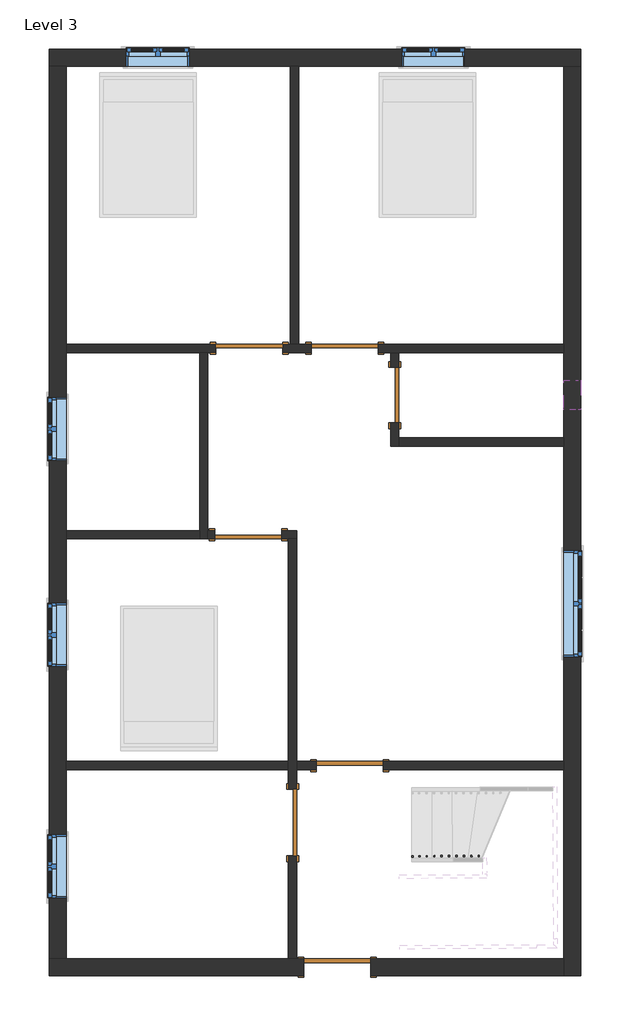
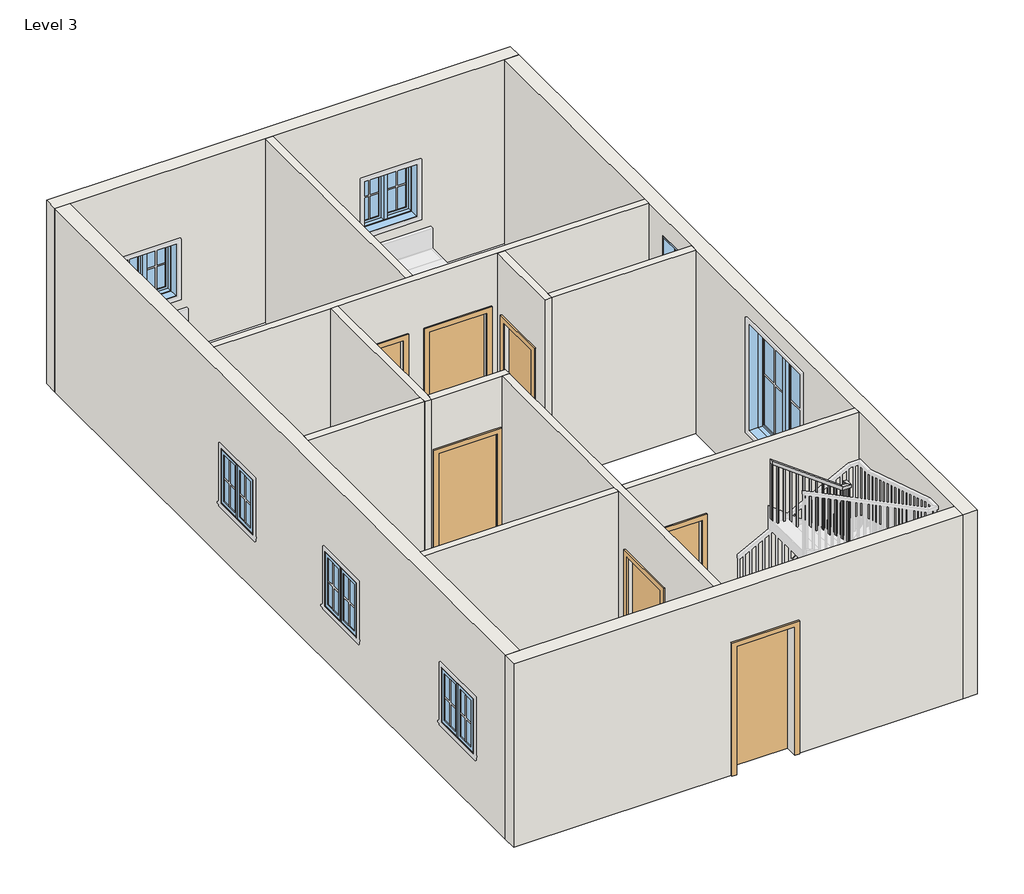
# One storey, part 1 of 2: 13 walls, 7 doors, 7 windows, 1 railing.
"""IFC4 building model written with IfcOpenShell, lengths in millimetres."""

from ifc_helpers import new_model, si_unit, frame, origin, place, context, project, spatial, polyline, outline, extrude, faceted_brep, transform, mapped, element, save
from components import door_f2b275c1, door_e5f9f3c4, door_305aa2a5, door_a90ba1ad, window_aa618e30, window_339605e1, window_9ac97e1a

model = new_model("IFC4")

# Units and contexts
model_context = context("Model", 3, world=origin())
ifc_project = project(units=[si_unit("LENGTHUNIT", "METRE", prefix="MILLI")], contexts=[model_context])

# Site, building, storey
site = spatial("IfcSite", under=ifc_project)
building = spatial("IfcBuilding", under=site)
storey = spatial("IfcBuildingStorey", under=building, Name="Level 3", Elevation=3200.4)

# Doors
placement = place(None, origin())
door_shape = door_f2b275c1(model_context)
element("IfcDoor", 1, ObjectType="Single-Flush : 30\" x 80\"", at=placement, inside=storey, context=model_context, shape_type="MappedRepresentation", body=[
    mapped(door_shape, transform((-163.0415084, 2144.7435985, 3200.4), x_axis=(0.0, 1.0, 0.0), y_axis=(-1.0, 0.0, 0.0), z_axis=(0.0, 0.0, 1.0))),
])
door_2_shape = door_e5f9f3c4(model_context)
element("IfcDoor", 2, ObjectType="Single-Flush : 36\" x 84\"", at=placement, inside=storey, context=model_context, shape_type="MappedRepresentation", body=[
    mapped(door_2_shape, transform((-2156.9415084, 2786.0935985, 3200.4), x_axis=(1.0, 0.0, 0.0), y_axis=(0.0, 1.0, 0.0), z_axis=(0.0, 0.0, 1.0))),
])
door_3_shape = door_305aa2a5(model_context)
element("IfcDoor", 3, ObjectType="Single-Flush : 36\" x 84\"", at=placement, inside=storey, context=model_context, shape_type="MappedRepresentation", body=[
    mapped(door_3_shape, transform((-848.8415084, 2786.0935985, 3200.4), x_axis=(-1.0, 0.0, 0.0), y_axis=(0.0, -1.0, 0.0), z_axis=(0.0, 0.0, 1.0))),
])
element("IfcDoor", 4, ObjectType="Single-Flush : 36\" x 84\"", at=placement, inside=storey, context=model_context, shape_type="MappedRepresentation", body=[
    mapped(door_3_shape, transform((-2170.1582019, 233.3935985, 3200.4), x_axis=(1.0, 0.0, 0.0), y_axis=(0.0, 1.0, 0.0), z_axis=(0.0, 0.0, 1.0))),
])
element("IfcDoor", 5, ObjectType="Single-Flush : 36\" x 84\"", at=placement, inside=storey, context=model_context, shape_type="MappedRepresentation", body=[
    mapped(door_3_shape, transform((-778.9915084, -2928.9064015, 3200.4), x_axis=(-1.0, 0.0, 0.0), y_axis=(0.0, -1.0, 0.0), z_axis=(0.0, 0.0, 1.0))),
])
element("IfcDoor", 6, ObjectType="Single-Flush : 36\" x 84\"", at=placement, inside=storey, context=model_context, shape_type="MappedRepresentation", body=[
    mapped(door_3_shape, transform((-1561.0748955, -3709.9564015, 3200.4), x_axis=(0.0, 1.0, 0.0), y_axis=(-1.0, 0.0, 0.0), z_axis=(0.0, 0.0, 1.0))),
])
door_4_shape = door_a90ba1ad(model_context)
element("IfcDoor", 7, ObjectType="Single-Flush : 36\" x 84\"", at=placement, inside=storey, context=model_context, shape_type="MappedRepresentation", body=[
    mapped(door_4_shape, transform((-951.4748955, -5691.1564015, 3200.4), x_axis=(-1.0, 0.0, 0.0), y_axis=(0.0, -1.0, 0.0), z_axis=(0.0, 0.0, 1.0))),
])

# Railing
element("IfcRailing", 8, ObjectType="Handrail - Rectangular", at=placement, inside=storey, context=model_context, shape_type="SolidModel", body=[
    faceted_brep([(73.2591805, -4146.3303197, 4792.1333333), (73.2591805, -4146.3303197, 4725.5495342), (73.5214139, -4197.1296428, 4725.5495342), (73.5214139, -4197.1296428, 4792.1333333), (1064.2769136, -4141.2145447, 5631.8511215), (1082.90463, -4141.1183857, 5581.0511215), (1083.1668634, -4191.9177089, 5581.0511215), (1064.5391469, -4192.0138678, 5631.8511215), (1144.655904, -4140.7996168, 5631.8511215), (1144.9181373, -4191.59894, 5631.8511215), (1144.9181373, -4191.59894, 5581.0511215), (1144.655904, -4140.7996168, 5581.0511215)], [[[0, 1, 2, 3]], [[1, 0, 4, 5]], [[2, 1, 5, 6]], [[3, 2, 6, 7]], [[0, 3, 7, 4]], [[8, 9, 10, 11]], [[5, 4, 8, 11]], [[6, 5, 11, 10]], [[7, 6, 10, 9]], [[4, 7, 9, 8]]]),
    faceted_brep([(1144.9181373, -4191.59894, 5640.3305642), (1144.9181373, -4191.59894, 5519.048826), (1094.1188142, -4191.8611734, 5519.048826), (1094.1188142, -4191.8611734, 5640.3305642), (1145.9670708, -4394.7962326, 6080.8506209), (1146.2293041, -4445.5955558, 6069.6988968), (1095.429981, -4445.8577892, 6069.6988968), (1095.1677476, -4395.058466, 6080.8506209), (1145.9670708, -4394.7962326, 6331.4424257), (1146.2293041, -4445.5955558, 6280.6424257), (1095.429981, -4445.8577892, 6280.6424257), (1095.1677476, -4395.058466, 6331.4424257), (1146.6226542, -4521.7945406, 6331.4424257), (1146.6226542, -4521.7945406, 6280.6424257), (1095.5610976, -4471.2574507, 6280.6424257), (1095.5610976, -4471.2574507, 6331.4424257), (1019.6243463, -4522.4501239, 6331.4424257), (1002.8333893, -4522.5368013, 6280.6424257), (1002.5711559, -4471.7374781, 6280.6424257), (1019.3621129, -4471.6508008, 6331.4424257), (-100.5579777, -4528.232665, 7162.8), (-100.8202111, -4477.4333418, 7162.8), (-100.8202111, -4477.4333418, 7099.5383775), (-100.5579777, -4528.232665, 7099.5383775)], [[[0, 1, 2, 3]], [[1, 0, 4, 5]], [[2, 1, 5, 6]], [[3, 2, 6, 7]], [[0, 3, 7, 4]], [[5, 4, 8, 9]], [[6, 5, 9, 10]], [[7, 6, 10, 11]], [[4, 7, 11, 8]], [[9, 8, 12, 13]], [[10, 9, 13, 14]], [[11, 10, 14, 15]], [[8, 11, 15, 12]], [[13, 12, 16, 17]], [[14, 13, 17, 18]], [[15, 14, 18, 19]], [[12, 15, 19, 16]], [[20, 21, 22, 23]], [[17, 16, 20, 23]], [[18, 17, 23, 22]], [[19, 18, 22, 21]], [[16, 19, 21, 20]]]),
    extrude(outline(polyline([(235.6690058, -19.05), (221.5309941, 0.0), (1247.144155, 0.0), (1247.144155, -19.05), (235.6690058, -19.05)])), frame((-107.5675843, -4512.3936381, 7326.2108217), z_axis=(-0.005162073969672187, 0.9999866764074069, 0.0), x_axis=(0.0, 0.0, -1.0)), (0.0, 0.0, 1.0), 19.05),
    extrude(outline(polyline([(235.6690059, -19.05), (221.5309942, 0.0), (1171.7414261, 0.0), (1171.7414261, -19.05), (235.6690059, -19.05)])), frame((-5.968938, -4511.8691714, 7250.8080928), z_axis=(-0.005162073969672187, 0.9999866764074069, 0.0), x_axis=(0.0, 0.0, -1.0)), (0.0, 0.0, 1.0), 19.05),
    extrude(outline(polyline([(235.6690058, -19.05), (221.5309941, 0.0), (1096.3386971, 0.0), (1096.3386971, -19.05), (235.6690058, -19.05)])), frame((95.6297083, -4511.3447046, 7175.4053638), z_axis=(-0.005162073969672187, 0.9999866764074069, 0.0), x_axis=(0.0, 0.0, -1.0)), (0.0, 0.0, 1.0), 19.05),
    extrude(outline(polyline([(235.6690059, -19.0499999), (221.5309942, 0.0), (1190.2693016, 0.0), (1190.2693016, -19.0499999), (235.6690059, -19.0499999)])), frame((197.2283547, -4510.8202379, 7100.0026349), z_axis=(-0.005162073969672187, 0.9999866764074069, 0.0), x_axis=(0.0, 0.0, -1.0)), (0.0, 0.0, 1.0), 19.05),
    extrude(outline(polyline([(235.6690058, -19.05), (221.5309942, 0.0), (1114.8665726, 0.0), (1114.8665726, -19.05), (235.6690058, -19.05)])), frame((298.827001, -4510.2957712, 7024.5999059), z_axis=(-0.005162073969672187, 0.9999866764074069, 0.0), x_axis=(0.0, 0.0, -1.0)), (0.0, 0.0, 1.0), 19.05),
    extrude(outline(polyline([(235.6690058, -19.05), (221.5309941, 0.0), (1039.4638436, 0.0), (1039.4638436, -19.05), (235.6690058, -19.05)])), frame((400.4256473, -4509.7713045, 6949.1971769), z_axis=(-0.005162073969672187, 0.9999866764074069, 0.0), x_axis=(0.0, 0.0, -1.0)), (0.0, 0.0, 1.0), 19.05),
    extrude(outline(polyline([(235.6690058, -19.05), (221.5309942, 0.0), (1133.394448, 0.0), (1133.394448, -19.05), (235.6690058, -19.05)])), frame((502.0242936, -4509.2468378, 6873.794448), z_axis=(-0.005162073969672187, 0.9999866764074069, 0.0), x_axis=(0.0, 0.0, -1.0)), (0.0, 0.0, 1.0), 19.05),
    extrude(outline(polyline([(235.6690058, -19.05), (221.5309941, 0.0), (1057.991719, 0.0), (1057.991719, -19.05), (235.6690058, -19.05)])), frame((603.6229399, -4508.7223711, 6798.391719), z_axis=(-0.005162073969672187, 0.9999866764074069, 0.0), x_axis=(0.0, 0.0, -1.0)), (0.0, 0.0, 1.0), 19.05),
    extrude(outline(polyline([(235.6690059, -19.05), (221.5309942, 0.0), (1151.9223234, 0.0), (1151.9223234, -19.05), (235.6690059, -19.05)])), frame((705.2215863, -4508.1979044, 6722.9889901), z_axis=(-0.005162073969672187, 0.9999866764074069, 0.0), x_axis=(0.0, 0.0, -1.0)), (0.0, 0.0, 1.0), 19.05),
    extrude(outline(polyline([(235.6690058, -19.05), (221.5309941, 0.0), (1076.5195944, 0.0), (1076.5195944, -19.05), (235.6690058, -19.05)])), frame((806.8202326, -4507.6734376, 6647.5862611), z_axis=(-0.005162073969672187, 0.9999866764074069, 0.0), x_axis=(0.0, 0.0, -1.0)), (0.0, 0.0, 1.0), 19.05),
    extrude(outline(polyline([(235.6690059, -19.05), (221.5309942, 0.0), (1170.4501989, 0.0), (1170.4501989, -19.05), (235.6690059, -19.05)])), frame((908.4188789, -4507.1489709, 6572.1835322), z_axis=(-0.005162073969672187, 0.9999866764074069, 0.0), x_axis=(0.0, 0.0, -1.0)), (0.0, 0.0, 1.0), 19.05),
    extrude(outline(polyline([(235.6690058, -19.05), (221.5309942, 0.0), (1095.0474699, 0.0), (1095.0474699, -19.05), (235.6690058, -19.05)])), frame((1010.0175252, -4506.6245042, 6496.7808032), z_axis=(-0.005162073969672187, 0.9999866764074069, 0.0), x_axis=(0.0, 0.0, -1.0)), (0.0, 0.0, 1.0), 19.05),
    extrude(outline(polyline([(1111.3867174, -4461.6506297), (1130.4364636, -4461.5522922), (1130.5348011, -4480.6020384), (1111.4850549, -4480.7003759), (1111.3867174, -4461.6506297)])), frame((0.0, 0.0, 5232.4), z_axis=(0.0, 0.0, 1.0), x_axis=(1.0, 0.0, 0.0)), (0.0, 0.0, 1.0), 1048.2424257),
    extrude(outline(polyline([(207.9506224, -19.05), (249.2493777, 0.0), (1070.0372089, 0.0), (1070.0372089, -19.05), (207.9506224, -19.05)])), frame((1110.8622507, -4360.0519834, 6133.1038756), z_axis=(0.9999866764074068, 0.005162073969671281, 0.0), x_axis=(0.0, 0.0, -1.0)), (0.0, 0.0, 1.0), 19.05),
    extrude(outline(polyline([(207.9506224, -19.05), (249.2493777, 0.0), (1019.110514, 0.0), (1019.110514, -19.05), (207.9506224, -19.05)])), frame((1110.3377839, -4258.4533371, 5912.8438473), z_axis=(0.9999866764074068, 0.005162073969671281, 0.0), x_axis=(0.0, 0.0, -1.0)), (0.0, 0.0, 1.0), 19.05),
    extrude(outline(polyline([(1079.9010561, -4176.0593559), (1079.8027186, -4157.0096098), (1098.8524648, -4156.9112722), (1098.9508023, -4175.9610184), (1079.9010561, -4176.0593559)])), frame((0.0, 0.0, 4555.0666667), z_axis=(0.0, 0.0, 1.0), x_axis=(1.0, 0.0, 0.0)), (0.0, 0.0, 1.0), 1025.9844548),
    extrude(outline(polyline([(220.5293015, -19.05), (236.6706986, 0.0), (1343.2032603, 0.0), (1343.2032603, -19.05), (220.5293015, -19.05)])), frame((978.3024098, -4176.5838227, 5728.9365936), z_axis=(-0.005162073969671482, 0.9999866764074068, 0.0), x_axis=(0.0, 0.0, -1.0)), (0.0, 0.0, 1.0), 19.05),
    extrude(outline(polyline([(220.5293015, -19.05), (236.6706985, 0.0), (1257.1158092, 0.0), (1257.1158092, -19.05), (220.5293015, -19.05)])), frame((876.7037635, -4177.1082894, 5642.8491425), z_axis=(-0.005162073969671482, 0.9999866764074068, 0.0), x_axis=(0.0, 0.0, -1.0)), (0.0, 0.0, 1.0), 19.05),
    extrude(outline(polyline([(220.5293015, -19.05), (236.6706986, 0.0), (1340.3616915, 0.0), (1340.3616915, -19.05), (220.5293015, -19.05)])), frame((775.1051171, -4177.6327561, 5556.7616915), z_axis=(-0.005162073969671482, 0.9999866764074068, 0.0), x_axis=(0.0, 0.0, -1.0)), (0.0, 0.0, 1.0), 19.05),
    extrude(outline(polyline([(220.5293014, -19.05), (236.6706985, 0.0), (1254.2742404, 0.0), (1254.2742404, -19.05), (220.5293014, -19.05)])), frame((673.5064708, -4178.1572228, 5470.6742404), z_axis=(-0.005162073969671482, 0.9999866764074068, 0.0), x_axis=(0.0, 0.0, -1.0)), (0.0, 0.0, 1.0), 19.05),
    extrude(outline(polyline([(220.5293015, -19.05), (236.6706985, 0.0), (1337.5201227, 0.0), (1337.5201227, -19.05), (220.5293015, -19.05)])), frame((571.9078245, -4178.6816895, 5384.5867894), z_axis=(-0.005162073969671482, 0.9999866764074068, 0.0), x_axis=(0.0, 0.0, -1.0)), (0.0, 0.0, 1.0), 19.05),
    extrude(outline(polyline([(220.5293015, -19.05), (236.6706986, 0.0), (1251.4326717, 0.0), (1251.4326717, -19.05), (220.5293015, -19.05)])), frame((470.3091782, -4179.2061562, 5298.4993384), z_axis=(-0.005162073969671482, 0.9999866764074068, 0.0), x_axis=(0.0, 0.0, -1.0)), (0.0, 0.0, 1.0), 19.05),
    extrude(outline(polyline([(220.5293014, -19.0499999), (236.6706985, 0.0), (1165.3452206, 0.0), (1165.3452206, -19.0499999), (220.5293014, -19.0499999)])), frame((368.7105319, -4179.7306229, 5212.4118873), z_axis=(-0.005162073969671482, 0.9999866764074068, 0.0), x_axis=(0.0, 0.0, -1.0)), (0.0, 0.0, 1.0), 19.05),
    extrude(outline(polyline([(220.5293015, -19.05), (236.6706986, 0.0), (1248.591103, 0.0), (1248.591103, -19.05), (220.5293015, -19.05)])), frame((267.1118855, -4180.2550897, 5126.3244363), z_axis=(-0.005162073969671482, 0.9999866764074068, 0.0), x_axis=(0.0, 0.0, -1.0)), (0.0, 0.0, 1.0), 19.05),
    extrude(outline(polyline([(220.5293014, -19.05), (236.6706985, 0.0), (1162.5036519, 0.0), (1162.5036519, -19.05), (220.5293014, -19.05)])), frame((165.5132392, -4180.7795564, 5040.2369852), z_axis=(-0.005162073969671482, 0.9999866764074068, 0.0), x_axis=(0.0, 0.0, -1.0)), (0.0, 0.0, 1.0), 19.05),
    extrude(outline(polyline([(1111.5178341, -4487.0502913), (1130.5675802, -4486.9519538), (1130.6659177, -4506.0017), (1111.6161716, -4506.1000375), (1111.5178341, -4487.0502913)])), frame((0.0, 0.0, 5232.4), z_axis=(0.0, 0.0, 1.0), x_axis=(1.0, 0.0, 0.0)), (0.0, 0.0, 1.0), 1048.2424257),
    extrude(outline(polyline([(1109.9116547, -4175.9044369), (1109.8133172, -4156.8546908), (1128.8630634, -4156.7563533), (1128.9614009, -4175.8060994), (1109.9116547, -4175.9044369)])), frame((0.0, 0.0, 4724.4), z_axis=(0.0, 0.0, 1.0), x_axis=(1.0, 0.0, 0.0)), (0.0, 0.0, 1.0), 856.6511215),
    extrude(outline(polyline([(235.6690058, -19.05), (221.5309941, 0.0), (1242.0027049, 0.0), (1242.0027049, -19.05), (235.6690058, -19.05)])), frame((-100.6399256, -4512.3578765, 7321.0693716), z_axis=(-0.005162073969672187, 0.9999866764074069, 0.0), x_axis=(0.0, 0.0, -1.0)), (0.0, 0.0, 1.0), 19.05),
    extrude(outline(polyline([(220.5293014, -19.05), (236.6706985, 0.0), (1084.4868994, 0.0), (1084.4868994, -19.05), (220.5293014, -19.05)])), frame((73.439466, -4181.2548543, 4962.2202327), z_axis=(-0.005162073969671482, 0.9999866764074068, 0.0), x_axis=(0.0, 0.0, -1.0)), (0.0, 0.0, 1.0), 19.05),
])

# Walls
element("IfcWall", 9, ObjectType="WALL4.5\"", at=placement, inside=storey, context=model_context, shape_type="Brep", body=[
    faceted_brep([(-1699.7415084, 2728.9435985, 3200.4), (-1306.0415084, 2728.9435985, 3200.4), (-1306.0415084, 2728.9435985, 5334.0), (-391.6415084, 2728.9435985, 5334.0), (-391.6415084, 2728.9435985, 3200.4), (-220.1915084, 2728.9435985, 3200.4), (-105.8915084, 2728.9435985, 3200.4), (2154.7084916, 2728.9435985, 3200.4), (2154.7084916, 2728.9435985, 6248.4), (-105.8915084, 2728.9435985, 6248.4), (-220.1915084, 2728.9435985, 6248.4), (-2722.0915084, 2728.9435985, 6248.4), (-2836.3915084, 2728.9435985, 6248.4), (-4665.1915084, 2728.9435985, 6248.4), (-4665.1915084, 2728.9435985, 3200.4), (-2836.3915084, 2728.9435985, 3200.4), (-2722.0915084, 2728.9435985, 3200.4), (-2614.1415084, 2728.9435985, 3200.4), (-2614.1415084, 2728.9435985, 5334.0), (-1699.7415084, 2728.9435985, 5334.0), (-1306.0415084, 2843.2435985, 5334.0), (-1306.0415084, 2843.2435985, 3200.4), (-1477.4915084, 2843.2435985, 3200.4), (-1591.7915084, 2843.2435985, 3200.4), (-1699.7415084, 2843.2435985, 3200.4), (-1699.7415084, 2843.2435985, 5334.0), (-2614.1415084, 2843.2435985, 5334.0), (-2614.1415084, 2843.2435985, 3200.4), (-4665.1915084, 2843.2435985, 3200.4), (-4665.1915084, 2843.2435985, 6248.4), (-1591.7915084, 2843.2435985, 6248.4), (-1477.4915084, 2843.2435985, 6248.4), (2154.7084916, 2843.2435985, 6248.4), (2154.7084916, 2843.2435985, 3200.4), (-391.6415084, 2843.2435985, 3200.4), (-391.6415084, 2843.2435985, 5334.0)], [[[0, 1, 2, 3, 4, 5, 6, 7, 8, 9, 10, 11, 12, 13, 14, 15, 16, 17, 18, 19]], [[20, 21, 22, 23, 24, 25, 26, 27, 28, 29, 30, 31, 32, 33, 34, 35]], [[17, 16, 15, 14, 28, 27]], [[34, 33, 7, 6, 5, 4]], [[24, 23, 22, 21, 1, 0]], [[8, 7, 33, 32]], [[14, 13, 29, 28]], [[25, 24, 0, 19]], [[26, 25, 19, 18]], [[27, 26, 18, 17]], [[2, 1, 21, 20]], [[3, 2, 20, 35]], [[4, 3, 35, 34]], [[13, 12, 11, 10, 9, 8, 32, 31, 30, 29]]]),
])
element("IfcWall", 10, ObjectType="WALL4.5\"", at=placement, inside=storey, context=model_context, shape_type="SweptSolid", body=[
    extrude(outline(polyline([(-1591.7915084, 2843.2435985), (-1591.7915084, 6653.2435985), (-1477.4915084, 6653.2435985), (-1477.4915084, 2843.2435985), (-1591.7915084, 2843.2435985)])), frame((0.0, 0.0, 3200.4), z_axis=(0.0, 0.0, 1.0), x_axis=(1.0, 0.0, 0.0)), (0.0, 0.0, 1.0), 3048.0),
])
element("IfcWall", 11, ObjectType="WALL4.5\"", at=placement, inside=storey, context=model_context, shape_type="Brep", body=[
    faceted_brep([(-2836.3915084, 2728.9435985, 3200.4), (-2836.3915084, 290.5435985, 3200.4), (-2836.3915084, 176.2435985, 3200.4), (-2836.3915084, 176.2435985, 6248.4), (-2836.3915084, 290.5435985, 6248.4), (-2836.3915084, 2728.9435985, 6248.4), (-2722.0915084, 2728.9435985, 3200.4), (-2722.0915084, 2728.9435985, 6248.4), (-2722.0915084, 290.5435985, 6248.4), (-2722.0915084, 176.2435985, 6248.4), (-2722.0915084, 176.2435985, 3200.4), (-2722.0915084, 290.5435985, 3200.4)], [[[0, 1, 2, 3, 4, 5]], [[6, 7, 8, 9, 10, 11]], [[2, 1, 0, 6, 11, 10]], [[0, 5, 7, 6]], [[3, 2, 10, 9]], [[5, 4, 3, 9, 8, 7]]]),
])
element("IfcWall", 12, ObjectType="WALL4.5\"", at=placement, inside=storey, context=model_context, shape_type="SweptSolid", body=[
    extrude(outline(polyline([(-2836.3915084, 176.2435985), (-4665.1915084, 176.2435985), (-4665.1915084, 290.5435985), (-2836.3915084, 290.5435985), (-2836.3915084, 176.2435985)])), frame((0.0, 0.0, 3200.4), z_axis=(0.0, 0.0, 1.0), x_axis=(1.0, 0.0, 0.0)), (0.0, 0.0, 1.0), 3048.0),
])
element("IfcWall", 13, ObjectType="WALL4.5\"", at=placement, inside=storey, context=model_context, shape_type="Brep", body=[
    faceted_brep([(-1712.9582019, 176.2435985, 5334.0), (-1712.9582019, 176.2435985, 3200.4), (-1618.2248955, 176.2435985, 3200.4), (-1503.9248955, 176.2435985, 3200.4), (-1502.8915084, 176.2435985, 3200.4), (-1502.8915084, 176.2435985, 6248.4), (-1503.9248955, 176.2435985, 6248.4), (-1618.2248955, 176.2435985, 6248.4), (-2722.0915084, 176.2435985, 6248.4), (-2722.0915084, 176.2435985, 3200.4), (-2627.3582019, 176.2435985, 3200.4), (-2627.3582019, 176.2435985, 5334.0), (-1502.8915084, 290.5435985, 3200.4), (-1712.9582019, 290.5435985, 3200.4), (-1712.9582019, 290.5435985, 5334.0), (-2627.3582019, 290.5435985, 5334.0), (-2627.3582019, 290.5435985, 3200.4), (-2722.0915084, 290.5435985, 3200.4), (-2722.0915084, 290.5435985, 6248.4), (-1502.8915084, 290.5435985, 6248.4)], [[[0, 1, 2, 3, 4, 5, 6, 7, 8, 9, 10, 11]], [[12, 13, 14, 15, 16, 17, 18, 19]], [[10, 9, 17, 16]], [[4, 3, 2, 1, 13, 12]], [[5, 4, 12, 19]], [[9, 8, 18, 17]], [[14, 13, 1, 0]], [[15, 14, 0, 11]], [[16, 15, 11, 10]], [[8, 7, 6, 5, 19, 18]]]),
])
element("IfcWall", 14, ObjectType="WALL4.5\"", at=placement, inside=storey, context=model_context, shape_type="Brep", body=[
    faceted_brep([(-1618.2248955, 176.2435985, 3200.4), (-1618.2248955, -2871.7564015, 3200.4), (-1618.2248955, -2986.0564015, 3200.4), (-1618.2248955, -3252.7564015, 3200.4), (-1618.2248955, -3252.7564015, 5334.0), (-1618.2248955, -4167.1564015, 5334.0), (-1618.2248955, -4167.1564015, 3200.4), (-1618.2248955, -5576.8564015, 3200.4), (-1618.2248955, -5576.8564015, 6248.4), (-1618.2248955, -2986.0564015, 6248.4), (-1618.2248955, -2871.7564015, 6248.4), (-1618.2248955, 176.2435985, 6248.4), (-1503.9248955, -3252.7564015, 5334.0), (-1503.9248955, -3252.7564015, 3200.4), (-1503.9248955, -2986.0564015, 3200.4), (-1503.9248955, -2871.7564015, 3200.4), (-1503.9248955, 176.2435985, 3200.4), (-1503.9248955, 176.2435985, 6248.4), (-1503.9248955, -2871.7564015, 6248.4), (-1503.9248955, -2986.0564015, 6248.4), (-1503.9248955, -5576.8564015, 6248.4), (-1503.9248955, -5576.8564015, 3200.4), (-1503.9248955, -4167.1564015, 3200.4), (-1503.9248955, -4167.1564015, 5334.0)], [[[0, 1, 2, 3, 4, 5, 6, 7, 8, 9, 10, 11]], [[12, 13, 14, 15, 16, 17, 18, 19, 20, 21, 22, 23]], [[22, 21, 7, 6]], [[16, 15, 14, 13, 3, 2, 1, 0]], [[8, 7, 21, 20]], [[0, 11, 17, 16]], [[4, 3, 13, 12]], [[5, 4, 12, 23]], [[6, 5, 23, 22]], [[11, 10, 9, 8, 20, 19, 18, 17]]]),
])
element("IfcWall", 15, ObjectType="WALL4.5\"", at=placement, inside=storey, context=model_context, shape_type="SweptSolid", body=[
    extrude(outline(polyline([(3200.4, 2154.7084916), (6248.4, 2154.7084916), (6248.4, -1503.9248955), (3200.4, -1503.9248955), (3200.4, -1236.1915084), (5334.0, -1236.1915084), (5334.0, -321.7915084), (3200.4, -321.7915084), (3200.4, 2154.7084916)])), frame((0.0, -2986.0564015, 0.0), z_axis=(0.0, 1.0, 0.0), x_axis=(0.0, 0.0, 1.0)), (0.0, 0.0, 1.0), 114.3),
    extrude(outline(polyline([(-4665.1915084, -2986.0564015), (-4665.1915084, -2871.7564015), (-1618.2248955, -2871.7564015), (-1618.2248955, -2986.0564015), (-4665.1915084, -2986.0564015)])), frame((0.0, 0.0, 3200.4), z_axis=(0.0, 0.0, 1.0), x_axis=(1.0, 0.0, 0.0)), (0.0, 0.0, 1.0), 3048.0),
])
element("IfcWall", 16, ObjectType="WALL4.5\"", at=placement, inside=storey, context=model_context, shape_type="Brep", body=[
    faceted_brep([(-220.1915084, 2728.9435985, 3200.4), (-220.1915084, 2525.7435985, 3200.4), (-220.1915084, 2525.7435985, 5232.4), (-220.1915084, 1763.7435985, 5232.4), (-220.1915084, 1763.7435985, 3200.4), (-220.1915084, 1446.2435985, 3200.4), (-220.1915084, 1446.2435985, 6248.4), (-220.1915084, 2728.9435985, 6248.4), (-105.8915084, 2525.7435985, 5232.4), (-105.8915084, 2525.7435985, 3200.4), (-105.8915084, 2728.9435985, 3200.4), (-105.8915084, 2728.9435985, 6248.4), (-105.8915084, 1560.5435985, 6248.4), (-105.8915084, 1446.2435985, 6248.4), (-105.8915084, 1446.2435985, 3200.4), (-105.8915084, 1560.5435985, 3200.4), (-105.8915084, 1763.7435985, 3200.4), (-105.8915084, 1763.7435985, 5232.4)], [[[0, 1, 2, 3, 4, 5, 6, 7]], [[8, 9, 10, 11, 12, 13, 14, 15, 16, 17]], [[10, 9, 1, 0]], [[16, 15, 14, 5, 4]], [[0, 7, 11, 10]], [[6, 5, 14, 13]], [[2, 1, 9, 8]], [[3, 2, 8, 17]], [[4, 3, 17, 16]], [[7, 6, 13, 12, 11]]]),
])
element("IfcWall", 17, ObjectType="WALL4.5\"", at=placement, inside=storey, context=model_context, shape_type="SweptSolid", body=[
    extrude(outline(polyline([(2154.7084916, 1446.2435985), (-105.8915084, 1446.2435985), (-105.8915084, 1560.5435985), (2154.7084916, 1560.5435985), (2154.7084916, 1446.2435985)])), frame((0.0, 0.0, 3200.4), z_axis=(0.0, 0.0, 1.0), x_axis=(1.0, 0.0, 0.0)), (0.0, 0.0, 1.0), 3048.0),
])
element("IfcWall", 18, ObjectType="WALL9\"", at=placement, inside=storey, context=model_context, shape_type="Brep", body=[
    faceted_brep([(-4893.7915084, 6653.2435985, 3200.4), (-4665.1915084, 6653.2435985, 3200.4), (-1591.7915084, 6653.2435985, 3200.4), (-1477.4915084, 6653.2435985, 3200.4), (2154.7084916, 6653.2435985, 3200.4), (2383.3084916, 6653.2435985, 3200.4), (2383.3084916, 6653.2435985, 6248.4), (2154.7084916, 6653.2435985, 6248.4), (-1477.4915084, 6653.2435985, 6248.4), (-1591.7915084, 6653.2435985, 6248.4), (-4665.1915084, 6653.2435985, 6248.4), (-4893.7915084, 6653.2435985, 6248.4), (-2976.0915084, 6653.2435985, 5029.2), (-2976.0915084, 6653.2435985, 4114.8), (-3839.6915084, 6653.2435985, 4114.8), (-3839.6915084, 6653.2435985, 5029.2), (798.9834916, 6653.2435985, 5029.2), (798.9834916, 6653.2435985, 4114.8), (-64.6165084, 6653.2435985, 4114.8), (-64.6165084, 6653.2435985, 5029.2), (-4893.7915084, 6881.8435985, 3200.4), (-4893.7915084, 6881.8435985, 6248.4), (2383.3084916, 6881.8435985, 6248.4), (2383.3084916, 6881.8435985, 3200.4), (-2976.0915084, 6881.8435985, 5029.2), (-3839.6915084, 6881.8435985, 5029.2), (-3839.6915084, 6881.8435985, 4114.8), (-2976.0915084, 6881.8435985, 4114.8), (798.9834916, 6881.8435985, 5029.2), (-64.6165084, 6881.8435985, 5029.2), (-64.6165084, 6881.8435985, 4114.8), (798.9834916, 6881.8435985, 4114.8)], [[[0, 1, 2, 3, 4, 5, 6, 7, 8, 9, 10, 11], [12, 13, 14, 15], [16, 17, 18, 19]], [[20, 21, 22, 23], [24, 25, 26, 27], [28, 29, 30, 31]], [[5, 4, 3, 2, 1, 0, 20, 23]], [[6, 5, 23, 22]], [[0, 11, 21, 20]], [[13, 12, 24, 27]], [[14, 13, 27, 26]], [[15, 14, 26, 25]], [[12, 15, 25, 24]], [[17, 16, 28, 31]], [[18, 17, 31, 30]], [[19, 18, 30, 29]], [[16, 19, 29, 28]], [[11, 10, 9, 8, 7, 6, 22, 21]]]),
])
element("IfcWall", 19, ObjectType="WALL9\"", at=placement, inside=storey, context=model_context, shape_type="Brep", body=[
    faceted_brep([(2154.7084916, 6653.2435985, 3200.4), (2154.7084916, 2843.2435985, 3200.4), (2154.7084916, 2728.9435985, 3200.4), (2154.7084916, 1560.5435985, 3200.4), (2154.7084916, 1446.2435985, 3200.4), (2154.7084916, -2871.7564015, 3200.4), (2154.7084916, -2986.0564015, 3200.4), (2154.7084916, -5576.8564015, 3200.4), (2154.7084916, -5805.4564015, 3200.4), (2154.7084916, -5805.4564015, 6248.4), (2154.7084916, -5576.8564015, 6248.4), (2154.7084916, -2986.0564015, 6248.4), (2154.7084916, -2871.7564015, 6248.4), (2154.7084916, 1446.2435985, 6248.4), (2154.7084916, 1560.5435985, 6248.4), (2154.7084916, 2728.9435985, 6248.4), (2154.7084916, 2843.2435985, 6248.4), (2154.7084916, 6653.2435985, 6248.4), (2154.7084916, 1941.5435985, 5943.6), (2154.7084916, 1941.5435985, 5334.0), (2154.7084916, 2347.9435985, 5334.0), (2154.7084916, 2347.9435985, 5943.6), (2154.7084916, -1436.6564015, 5943.6), (2154.7084916, -1436.6564015, 4114.8), (2154.7084916, 11.1435985, 4114.8), (2154.7084916, 11.1435985, 5943.6), (2383.3084916, 6653.2435985, 3200.4), (2383.3084916, 6653.2435985, 6248.4), (2383.3084916, -5805.4564015, 6248.4), (2383.3084916, -5805.4564015, 3200.4), (2383.3084916, 1941.5435985, 5943.6), (2383.3084916, 2347.9435985, 5943.6), (2383.3084916, 2347.9435985, 5334.0), (2383.3084916, 1941.5435985, 5334.0), (2383.3084916, -1436.6564015, 5943.6), (2383.3084916, 11.1435985, 5943.6), (2383.3084916, 11.1435985, 4114.8), (2383.3084916, -1436.6564015, 4114.8)], [[[0, 1, 2, 3, 4, 5, 6, 7, 8, 9, 10, 11, 12, 13, 14, 15, 16, 17], [18, 19, 20, 21], [22, 23, 24, 25]], [[26, 27, 28, 29], [30, 31, 32, 33], [34, 35, 36, 37]], [[8, 7, 6, 5, 4, 3, 2, 1, 0, 26, 29]], [[0, 17, 27, 26]], [[9, 8, 29, 28]], [[19, 18, 30, 33]], [[20, 19, 33, 32]], [[21, 20, 32, 31]], [[18, 21, 31, 30]], [[23, 22, 34, 37]], [[24, 23, 37, 36]], [[25, 24, 36, 35]], [[22, 25, 35, 34]], [[17, 16, 15, 14, 13, 12, 11, 10, 9, 28, 27]]]),
])
element("IfcWall", 20, ObjectType="WALL9\"", at=placement, inside=storey, context=model_context, shape_type="Brep", body=[
    faceted_brep([(-1408.6748955, -5576.8564015, 5334.0), (-1408.6748955, -5576.8564015, 3200.4), (-1503.9248955, -5576.8564015, 3200.4), (-1618.2248955, -5576.8564015, 3200.4), (-4665.1915084, -5576.8564015, 3200.4), (-4893.7915084, -5576.8564015, 3200.4), (-4893.7915084, -5576.8564015, 6248.4), (-4665.1915084, -5576.8564015, 6248.4), (-1618.2248955, -5576.8564015, 6248.4), (-1503.9248955, -5576.8564015, 6248.4), (2154.7084916, -5576.8564015, 6248.4), (2154.7084916, -5576.8564015, 3200.4), (-494.2748955, -5576.8564015, 3200.4), (-494.2748955, -5576.8564015, 5334.0), (-4893.7915084, -5805.4564015, 3200.4), (-1408.6748955, -5805.4564015, 3200.4), (-1408.6748955, -5805.4564015, 5334.0), (-494.2748955, -5805.4564015, 5334.0), (-494.2748955, -5805.4564015, 3200.4), (2154.7084916, -5805.4564015, 3200.4), (2154.7084916, -5805.4564015, 6248.4), (-4893.7915084, -5805.4564015, 6248.4)], [[[0, 1, 2, 3, 4, 5, 6, 7, 8, 9, 10, 11, 12, 13]], [[14, 15, 16, 17, 18, 19, 20, 21]], [[12, 11, 19, 18]], [[5, 4, 3, 2, 1, 15, 14]], [[11, 10, 20, 19]], [[6, 5, 14, 21]], [[16, 15, 1, 0]], [[17, 16, 0, 13]], [[18, 17, 13, 12]], [[10, 9, 8, 7, 6, 21, 20]]]),
])
element("IfcWall", 21, ObjectType="WALL9\"", at=placement, inside=storey, context=model_context, shape_type="Brep", body=[
    faceted_brep([(-4665.1915084, -5576.8564015, 3200.4), (-4665.1915084, -2986.0564015, 3200.4), (-4665.1915084, -2871.7564015, 3200.4), (-4665.1915084, 176.2435985, 3200.4), (-4665.1915084, 290.5435985, 3200.4), (-4665.1915084, 2728.9435985, 3200.4), (-4665.1915084, 2843.2435985, 3200.4), (-4665.1915084, 6653.2435985, 3200.4), (-4665.1915084, 6653.2435985, 6248.4), (-4665.1915084, 2843.2435985, 6248.4), (-4665.1915084, 2728.9435985, 6248.4), (-4665.1915084, 290.5435985, 6248.4), (-4665.1915084, 176.2435985, 6248.4), (-4665.1915084, -2871.7564015, 6248.4), (-4665.1915084, -2986.0564015, 6248.4), (-4665.1915084, -5576.8564015, 6248.4), (-4665.1915084, 2112.9935985, 5029.2), (-4665.1915084, 2112.9935985, 4114.8), (-4665.1915084, 1249.3935985, 4114.8), (-4665.1915084, 1249.3935985, 5029.2), (-4665.1915084, -706.4064015, 5029.2), (-4665.1915084, -706.4064015, 4114.8), (-4665.1915084, -1570.0064015, 4114.8), (-4665.1915084, -1570.0064015, 5029.2), (-4665.1915084, -3878.2314015, 5029.2), (-4665.1915084, -3878.2314015, 4114.8), (-4665.1915084, -4741.8314015, 4114.8), (-4665.1915084, -4741.8314015, 5029.2), (-4893.7915084, -5576.8564015, 3200.4), (-4893.7915084, -5576.8564015, 6248.4), (-4893.7915084, 6653.2435985, 6248.4), (-4893.7915084, 6653.2435985, 3200.4), (-4893.7915084, 2112.9935985, 5029.2), (-4893.7915084, 1249.3935985, 5029.2), (-4893.7915084, 1249.3935985, 4114.8), (-4893.7915084, 2112.9935985, 4114.8), (-4893.7915084, -706.4064015, 5029.2), (-4893.7915084, -1570.0064015, 5029.2), (-4893.7915084, -1570.0064015, 4114.8), (-4893.7915084, -706.4064015, 4114.8), (-4893.7915084, -3878.2314015, 5029.2), (-4893.7915084, -4741.8314015, 5029.2), (-4893.7915084, -4741.8314015, 4114.8), (-4893.7915084, -3878.2314015, 4114.8)], [[[0, 1, 2, 3, 4, 5, 6, 7, 8, 9, 10, 11, 12, 13, 14, 15], [16, 17, 18, 19], [20, 21, 22, 23], [24, 25, 26, 27]], [[28, 29, 30, 31], [32, 33, 34, 35], [36, 37, 38, 39], [40, 41, 42, 43]], [[7, 6, 5, 4, 3, 2, 1, 0, 28, 31]], [[0, 15, 29, 28]], [[8, 7, 31, 30]], [[17, 16, 32, 35]], [[18, 17, 35, 34]], [[19, 18, 34, 33]], [[16, 19, 33, 32]], [[21, 20, 36, 39]], [[22, 21, 39, 38]], [[23, 22, 38, 37]], [[20, 23, 37, 36]], [[25, 24, 40, 43]], [[26, 25, 43, 42]], [[27, 26, 42, 41]], [[24, 27, 41, 40]], [[15, 14, 13, 12, 11, 10, 9, 8, 30, 29]]]),
])

# Windows
window_shape = window_aa618e30(model_context)
element("IfcWindow", 22, ObjectType="Fixed : 16\" x 24\"", at=placement, inside=storey, context=model_context, shape_type="MappedRepresentation", body=[
    mapped(window_shape, transform((2269.0084916, 2106.6435985, 4419.6), x_axis=(0.0, -1.0, 0.0), y_axis=(1.0, 0.0, 0.0), z_axis=(0.0, 0.0, 1.0))),
])
window_2_shape = window_339605e1(model_context)
element("IfcWindow", 23, ObjectType="Window-Casement-Double : 34\" x 36\"", at=placement, inside=storey, context=model_context, shape_type="MappedRepresentation", body=[
    mapped(window_2_shape, transform((-3407.8915084, 6767.5435985, 3200.4), x_axis=(1.0, 0.0, 0.0), y_axis=(0.0, 1.0, 0.0), z_axis=(0.0, 0.0, 1.0))),
])
element("IfcWindow", 24, ObjectType="Window-Casement-Double : 34\" x 36\"", at=placement, inside=storey, context=model_context, shape_type="MappedRepresentation", body=[
    mapped(window_2_shape, transform((367.1834916, 6767.5435985, 3200.4), x_axis=(1.0, 0.0, 0.0), y_axis=(0.0, 1.0, 0.0), z_axis=(0.0, 0.0, 1.0))),
])
element("IfcWindow", 25, ObjectType="Window-Casement-Double : 34\" x 36\"", at=placement, inside=storey, context=model_context, shape_type="MappedRepresentation", body=[
    mapped(window_2_shape, transform((-4779.4915084, 1681.1935985, 3200.4), x_axis=(0.0, 1.0, 0.0), y_axis=(-1.0, 0.0, 0.0), z_axis=(0.0, 0.0, 1.0))),
])
element("IfcWindow", 26, ObjectType="Window-Casement-Double : 34\" x 36\"", at=placement, inside=storey, context=model_context, shape_type="MappedRepresentation", body=[
    mapped(window_2_shape, transform((-4779.4915084, -1138.2064015, 3200.4), x_axis=(0.0, 1.0, 0.0), y_axis=(-1.0, 0.0, 0.0), z_axis=(0.0, 0.0, 1.0))),
])
element("IfcWindow", 27, ObjectType="Window-Casement-Double : 34\" x 36\"", at=placement, inside=storey, context=model_context, shape_type="MappedRepresentation", body=[
    mapped(window_2_shape, transform((-4779.4915084, -4310.0314015, 3200.4), x_axis=(0.0, 1.0, 0.0), y_axis=(-1.0, 0.0, 0.0), z_axis=(0.0, 0.0, 1.0))),
])
window_3_shape = window_9ac97e1a(model_context)
element("IfcWindow", 28, ObjectType="Window-Casement-Double : 57\" x 72\"", at=placement, inside=storey, context=model_context, shape_type="MappedRepresentation", body=[
    mapped(window_3_shape, transform((2269.0084916, -712.7564015, 3200.4), x_axis=(0.0, -1.0, 0.0), y_axis=(1.0, 0.0, 0.0), z_axis=(0.0, 0.0, 1.0))),
])

save(model, "model.ifc")

# Revit data of these elements
# Type "Single-Flush : 30\" x 80\""
#   Type Mark = "5"
#   Construction Type Id = "MDOOR"
#   Assembly Code = "C1020"
#   Analytic Construction = "Metal"
#   Thickness = 0' - 2"
#   Heat Transfer Coefficient (U) = 0.651978 BTU/(h·ft²·°F)
#   Height = 6' - 8"
#   Trim Projection Ext = 0' - 1"
#   Trim Projection Int = 0' - 1"
#   Trim Width = 0' - 3"
#   Width = 2' - 6"
#   Define Thermal Properties by = 1
#   Define Thermal Properties by = 1
#   Door Material = Door - Panel
#   Frame Material = Door - Frame
#   Visual Light Transmittance = 0
#   Solar Heat Gain Coefficient = 0
#   Function = (empty or 0)
#   Wall Closure = (empty or 0)
# Type "Single-Flush : 36\" x 84\""
#   Type Mark = "1"
#   Construction Type Id = "MDOOR"
#   Assembly Code = "C1020"
#   Analytic Construction = "Metal"
#   Thickness = 0' - 2"
#   Heat Transfer Coefficient (U) = 0.651978 BTU/(h·ft²·°F)
#   Height = 7' - 0"
#   Trim Projection Ext = 0' - 1"
#   Trim Projection Int = 0' - 1"
#   Trim Width = 0' - 3"
#   Width = 3' - 0"
#   Define Thermal Properties by = 1
#   Define Thermal Properties by = 1
#   Door Material = Door - Panel
#   Frame Material = Door - Frame
#   Visual Light Transmittance = 0
#   Solar Heat Gain Coefficient = 0
#   Function = (empty or 0)
#   Wall Closure = (empty or 0)
# Type "Handrail - Rectangular"
#   Assembly Code = "C2010400"
#   built-in parameter 1008612 = 0.0416667 (stored number, unit not read)
#   built-in parameter 1008611 = 0.0416667 (stored number, unit not read)
#   built-in parameter 1008609 = 0.333333 (stored number, unit not read)
#   built-in parameter 1008604 = 0.166667 (stored number, unit not read)
#   built-in parameter 1008603 = 0.166667 (stored number, unit not read)
#   Railing Height = 3' - 0"
#   built-in parameter 1008630 = 2
#   built-in parameter 1008610 = 2
#   built-in parameter 1008618 = Baluster - Square : 3/4"
# Type "WALL4.5\""
#   Assembly Code = "B2010"
#   Layers, outside or top first: 0' - 4 1/2" no material (function 1)
# Type "WALL9\""
#   Assembly Code = "B2010"
#   Layers, outside or top first: 0' - 9" no material (function 1)
# Type "Fixed : 16\" x 24\""
#   Type Mark = "4"
#   Construction Type Id = "GSP4R"
#   Assembly Code = "B2020100"
#   Analytic Construction = "1/8 in Pilkington single glazing"
#   Visual Light Transmittance = 0.9
#   Solar Heat Gain Coefficient = 0.78
#   Heat Transfer Coefficient (U) = 0.6496 BTU/(h·ft²·°F)
#   Height = 2' - 0"
#   Default Sill Height = 3' - 0"
#   Width = 1' - 4"
#   Window Inset = 0' - 0 3/4"
#   Define Thermal Properties by = 1
#   Define Thermal Properties by = 1
#   Glass Pane Material = Glass
#   Sash Material = Sash
#   Wall Closure = (empty or 0)
# Type "Window-Casement-Double : 34\" x 36\""
#   Type Mark = "14"
#   Fire Rating = "0.5h"
#   Assembly Code = "B2020100"
#   Analytic Construction = "Double glazing - domestic"
#   Frame Extension [instance default] = 0' - 0 1/4"
#   Window Inset [instance default] = 0' - 0"
#   Wall Thickness [instance default] = 0' - 6"
#   Interior Wall Closure [instance default] = 0' - 2 1/4"
#   Half Width = 1' - 5"
#   Visual Light Transmittance = 0.81
#   Thermal Resistance (R) = 1.8146 (h·ft²·°F)/BTU
#   Solar Heat Gain Coefficient = 0.76
#   Rough Width = 2' - 10 1/2"
#   Rough Height = 3' - 0 1/2"
#   Height = 3' - 0"
#   Heat Transfer Coefficient (U) = 0.5511 BTU/(h·ft²·°F)
#   Exterior Wall Closure [instance default] = 0' - 1 1/4"
#   Extension Jamb [instance default] = 0' - 2 1/4"
#   Default Sill Height = 3' - 0"
#   Width = 2' - 10"
#   Define Thermal Properties by = 0
#   Muntin Visibility = yes
#   Interior Trim Visibility [instance default] = yes
#   Exterior Trim Visibility [instance default] = yes
#   Extension Jamb Visibility [instance default] = yes
#   Interior Trim Material = Wood - Stained
#   Muntin Pattern = Muntin Pattern_2x2 : Muntin Pattern_2x2
#   Interior Trim = Trim-Window-Interior-Flat : Picture Frame
#   Interior Frame Material = Wood - Stained
#   Glass Panel Material = Glass
#   Exterior Trim Material = Clad - White
#   Exterior Trim = Trim-Window-Exterior-Flat : with Sill
#   Exterior Frame Material = Clad - White
#   Wall Closure = (empty or 0)
# Type "Window-Casement-Double : 57\" x 72\""
#   Type Mark = "17"
#   Fire Rating = "0.5h"
#   Assembly Code = "B2020100"
#   Analytic Construction = "Double glazing - domestic"
#   Frame Extension [instance default] = 0' - 0 1/4"
#   Window Inset [instance default] = 0' - 0"
#   Wall Thickness [instance default] = 0' - 6"
#   Interior Wall Closure [instance default] = 0' - 2 1/4"
#   Half Width = 2' - 4 1/2"
#   Visual Light Transmittance = 0.81
#   Thermal Resistance (R) = 1.8146 (h·ft²·°F)/BTU
#   Solar Heat Gain Coefficient = 0.76
#   Rough Width = 4' - 9 1/2"
#   Rough Height = 6' - 0 1/2"
#   Height = 6' - 0"
#   Heat Transfer Coefficient (U) = 0.5511 BTU/(h·ft²·°F)
#   Exterior Wall Closure [instance default] = 0' - 1 1/4"
#   Extension Jamb [instance default] = 0' - 2 1/4"
#   Default Sill Height = 3' - 0"
#   Width = 4' - 9"
#   Define Thermal Properties by = 0
#   Muntin Visibility = yes
#   Interior Trim Visibility [instance default] = yes
#   Exterior Trim Visibility [instance default] = yes
#   Extension Jamb Visibility [instance default] = yes
#   Interior Trim Material = Wood - Stained
#   Muntin Pattern = Muntin Pattern_2x2 : Muntin Pattern_2x2
#   Interior Trim = Trim-Window-Interior-Flat : Picture Frame
#   Interior Frame Material = Wood - Stained
#   Glass Panel Material = Glass
#   Exterior Trim Material = Clad - White
#   Exterior Trim = Trim-Window-Exterior-Flat : with Sill
#   Exterior Frame Material = Clad - White
#   Wall Closure = (empty or 0)
# Element 1 (IfcDoor, "Single-Flush : 30\" x 80\"")
#   Phase Created = New Construction
#   Materials on its faces: "Door - Frame", "Door - Panel"
# Elements 2, 3, 4, 5, 6, 7 (IfcDoor, "Single-Flush : 36\" x 84\"")
#   Phase Created = New Construction
#   Materials on its faces: "Door - Frame", "Door - Panel"
# Element 8 (IfcRailing, "Handrail - Rectangular")
#   Phase Created = New Construction
# Elements 9, 10, 11, 12, 13, 14, 15, 16, 17 (IfcWall, "WALL4.5\"")
#   Top Offset = 0' - 0"
#   Base Offset = 0' - 0"
#   Unconnected Height = 10' - 0"
#   wall height = 10' - 0"
#   Phase Created = New Construction
#   Base Constraint = Level 3
#   Materials on its faces: "Default Wall"
# Elements 18, 19, 20, 21 (IfcWall, "WALL9\"")
#   Top Offset = 0' - 0"
#   Base Offset = 0' - 0"
#   Unconnected Height = 10' - 0"
#   wall height = 10' - 0"
#   Phase Created = New Construction
#   Base Constraint = Level 3
#   Materials on its faces: "Default Wall", "Door - Frame"
# Element 22 (IfcWindow, "Fixed : 16\" x 24\"")
#   Mark = "9"
#   Phase Created = New Construction
#   Materials on its faces: "Sash", "Glass"
# Element 23 (IfcWindow, "Window-Casement-Double : 34\" x 36\"")
#   Mark = "10"
#   Window Inset = 0' - 0"
#   Interior Wall Closure = 0' - 2 1/4"
#   Frame Extension = 0' - 0 1/4"
#   Exterior Wall Closure = 0' - 1 1/4"
#   Interior Trim Visibility = yes
#   Exterior Trim Visibility = yes
#   Phase Created = New Construction
#   Materials on its faces: "Wood - Stained", "Glass", "Clad - White"
# Element 24 (IfcWindow, "Window-Casement-Double : 34\" x 36\"")
#   Mark = "11"
#   Window Inset = 0' - 0"
#   Interior Wall Closure = 0' - 2 1/4"
#   Frame Extension = 0' - 0 1/4"
#   Exterior Wall Closure = 0' - 1 1/4"
#   Interior Trim Visibility = yes
#   Exterior Trim Visibility = yes
#   Phase Created = New Construction
#   Materials on its faces: "Wood - Stained", "Glass", "Clad - White"
# Element 25 (IfcWindow, "Window-Casement-Double : 34\" x 36\"")
#   Mark = "12"
#   Window Inset = 0' - 0"
#   Interior Wall Closure = 0' - 2 1/4"
#   Frame Extension = 0' - 0 1/4"
#   Exterior Wall Closure = 0' - 1 1/4"
#   Interior Trim Visibility = yes
#   Exterior Trim Visibility = yes
#   Phase Created = New Construction
#   Materials on its faces: "Wood - Stained", "Glass", "Clad - White"
# Element 26 (IfcWindow, "Window-Casement-Double : 34\" x 36\"")
#   Mark = "13"
#   Window Inset = 0' - 0"
#   Interior Wall Closure = 0' - 2 1/4"
#   Frame Extension = 0' - 0 1/4"
#   Exterior Wall Closure = 0' - 1 1/4"
#   Interior Trim Visibility = yes
#   Exterior Trim Visibility = yes
#   Phase Created = New Construction
#   Materials on its faces: "Wood - Stained", "Glass", "Clad - White"
# Element 27 (IfcWindow, "Window-Casement-Double : 34\" x 36\"")
#   Mark = "14"
#   Window Inset = 0' - 0"
#   Interior Wall Closure = 0' - 2 1/4"
#   Frame Extension = 0' - 0 1/4"
#   Exterior Wall Closure = 0' - 1 1/4"
#   Interior Trim Visibility = yes
#   Exterior Trim Visibility = yes
#   Phase Created = New Construction
#   Materials on its faces: "Wood - Stained", "Glass", "Clad - White"
# Element 28 (IfcWindow, "Window-Casement-Double : 57\" x 72\"")
#   Mark = "15"
#   Window Inset = 0' - 0"
#   Interior Wall Closure = 0' - 2 1/4"
#   Frame Extension = 0' - 0 1/4"
#   Exterior Wall Closure = 0' - 1 1/4"
#   Interior Trim Visibility = yes
#   Exterior Trim Visibility = yes
#   Phase Created = New Construction
#   Materials on its faces: "Wood - Stained", "Glass", "Clad - White"
# Materials
#   "Door - Panel": class "Wood", colour RGB 210 159 95, transparency 0, Cost = 0
#   "Door - Frame": colour RGB 118 70 51, transparency 0, Cost = 0
#   "Glass": class "Glass", colour RGB 0 128 192, transparency 0.75, Description = "Soda Lime Glass", Cost = 0
#   "Sash": class "Wood", colour RGB 224 178 126, transparency 0, Cost = 0
#   "Wood - Stained": class "Wood", colour RGB 224 178 126, transparency 0, Cost = 0
#   "Clad - White": class "Wood", colour RGB 242 242 238, transparency 0, Cost = 0
#   "Default Wall": colour RGB 128 128 128, transparency 0, Cost = 0
